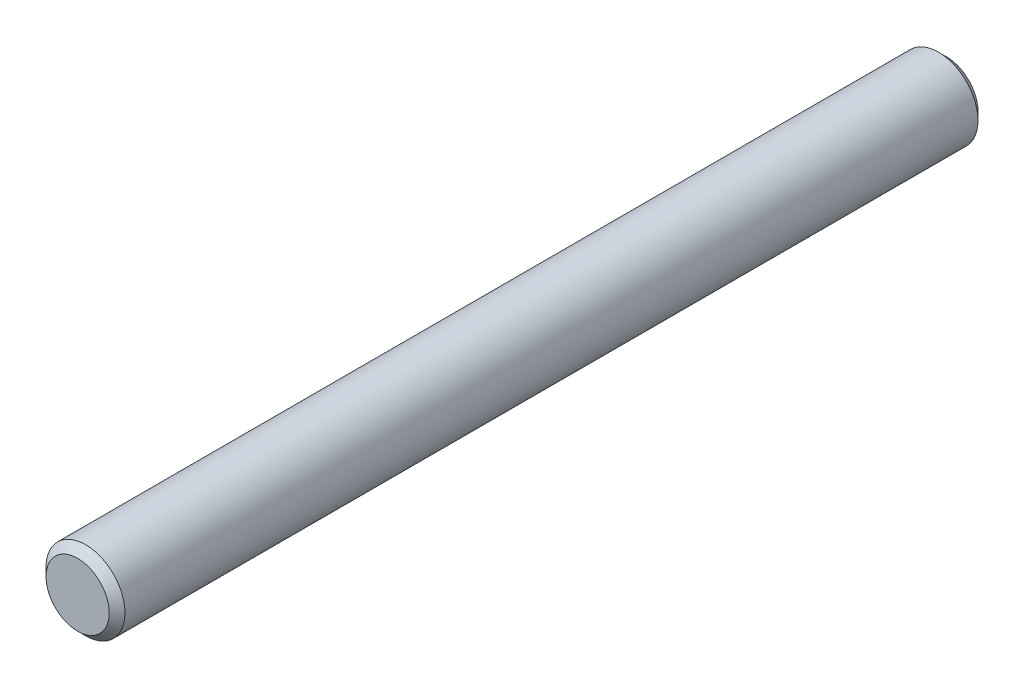
ISO-10303-21;
HEADER;
FILE_DESCRIPTION(('STEP AP214'),'2;1');
FILE_NAME('part.step','',(''),(''),'','','');
FILE_SCHEMA(('AUTOMOTIVE_DESIGN { 1 0 10303 214 1 1 1 1 }'));
ENDSEC;
DATA;
#1=APPLICATION_CONTEXT('core data for automotive mechanical design processes');
#2=APPLICATION_PROTOCOL_DEFINITION('international standard','automotive_design',2000,#1);
#3=PRODUCT_CONTEXT('',#1,'mechanical');
#4=PRODUCT('Part','Part','',(#3));
#5=PRODUCT_RELATED_PRODUCT_CATEGORY('part','',(#4));
#6=PRODUCT_DEFINITION_FORMATION('','',#4);
#7=PRODUCT_DEFINITION_CONTEXT('part definition',#1,'design');
#8=PRODUCT_DEFINITION('design','',#6,#7);
#9=PRODUCT_DEFINITION_SHAPE('','',#8);
#10=(LENGTH_UNIT() NAMED_UNIT(*) SI_UNIT(.MILLI.,.METRE.));
#11=(NAMED_UNIT(*) PLANE_ANGLE_UNIT() SI_UNIT($,.RADIAN.));
#12=(NAMED_UNIT(*) SI_UNIT($,.STERADIAN.) SOLID_ANGLE_UNIT());
#13=UNCERTAINTY_MEASURE_WITH_UNIT(LENGTH_MEASURE(1.E-05),#10,'distance_accuracy_value','');
#14=(GEOMETRIC_REPRESENTATION_CONTEXT(3) GLOBAL_UNCERTAINTY_ASSIGNED_CONTEXT((#13)) GLOBAL_UNIT_ASSIGNED_CONTEXT((#10,
#11,#12)) REPRESENTATION_CONTEXT('',''));
#15=CARTESIAN_POINT('',(0.,0.,0.));
#16=DIRECTION('',(0.,0.,1.));
#17=DIRECTION('',(1.,0.,0.));
#18=AXIS2_PLACEMENT_3D('',#15,#16,#17);
#19=CARTESIAN_POINT('',(0.,0.,27.5));
#20=DIRECTION('',(0.,0.,-1.));
#21=DIRECTION('',(-1.,0.,0.));
#22=AXIS2_PLACEMENT_3D('',#19,#20,#21);
#23=CYLINDRICAL_SURFACE('',#22,2.5);
#24=CARTESIAN_POINT('',(0.,0.,-27.));
#25=DIRECTION('',(0.,0.,1.));
#26=DIRECTION('',(1.,0.,0.));
#27=AXIS2_PLACEMENT_3D('',#24,#25,#26);
#28=CIRCLE('',#27,2.5);
#29=CARTESIAN_POINT('',(2.5,0.,-27.));
#30=VERTEX_POINT('',#29);
#31=EDGE_CURVE('E52',#30,#30,#28,.T.);
#32=ORIENTED_EDGE('',*,*,#31,.T.);
#33=EDGE_LOOP('',(#32));
#34=FACE_BOUND('',#33,.T.);
#35=CARTESIAN_POINT('',(0.,0.,27.));
#36=DIRECTION('',(0.,0.,1.));
#37=DIRECTION('',(1.,0.,0.));
#38=AXIS2_PLACEMENT_3D('',#35,#36,#37);
#39=CIRCLE('',#38,2.5);
#40=CARTESIAN_POINT('',(2.5,0.,27.));
#41=VERTEX_POINT('',#40);
#42=EDGE_CURVE('E60',#41,#41,#39,.F.);
#43=ORIENTED_EDGE('',*,*,#42,.T.);
#44=EDGE_LOOP('',(#43));
#45=FACE_BOUND('',#44,.T.);
#46=ADVANCED_FACE('F41',(#34,#45),#23,.T.);
#47=CARTESIAN_POINT('',(0.,0.,27.5));
#48=DIRECTION('',(0.,0.,1.));
#49=DIRECTION('',(1.,0.,0.));
#50=AXIS2_PLACEMENT_3D('',#47,#48,#49);
#51=PLANE('',#50);
#52=CARTESIAN_POINT('',(0.,0.,27.5));
#53=DIRECTION('',(0.,0.,1.));
#54=DIRECTION('',(1.,0.,0.));
#55=AXIS2_PLACEMENT_3D('',#52,#53,#54);
#56=CIRCLE('',#55,1.99999999999998);
#57=CARTESIAN_POINT('',(1.99999999999998,0.,27.5));
#58=VERTEX_POINT('',#57);
#59=EDGE_CURVE('E10',#58,#58,#56,.T.);
#60=ORIENTED_EDGE('',*,*,#59,.T.);
#61=EDGE_LOOP('',(#60));
#62=FACE_BOUND('',#61,.T.);
#63=ADVANCED_FACE('F71',(#62),#51,.T.);
#64=CARTESIAN_POINT('',(0.,0.,-27.5));
#65=DIRECTION('',(0.,0.,1.));
#66=DIRECTION('',(1.,0.,0.));
#67=AXIS2_PLACEMENT_3D('',#64,#65,#66);
#68=PLANE('',#67);
#69=CARTESIAN_POINT('',(0.,0.,-27.5));
#70=DIRECTION('',(0.,0.,1.));
#71=DIRECTION('',(1.,0.,0.));
#72=AXIS2_PLACEMENT_3D('',#69,#70,#71);
#73=CIRCLE('',#72,2.);
#74=CARTESIAN_POINT('',(2.,0.,-27.5));
#75=VERTEX_POINT('',#74);
#76=EDGE_CURVE('E47',#75,#75,#73,.F.);
#77=ORIENTED_EDGE('',*,*,#76,.T.);
#78=EDGE_LOOP('',(#77));
#79=FACE_BOUND('',#78,.T.);
#80=ADVANCED_FACE('F69',(#79),#68,.F.);
#81=CARTESIAN_POINT('',(0.,0.,-27.));
#82=DIRECTION('',(0.,0.,1.));
#83=DIRECTION('',(1.,0.,0.));
#84=AXIS2_PLACEMENT_3D('',#81,#82,#83);
#85=CONICAL_SURFACE('',#84,2.5,0.785398163397453);
#86=ORIENTED_EDGE('',*,*,#76,.F.);
#87=EDGE_LOOP('',(#86));
#88=FACE_BOUND('',#87,.T.);
#89=ORIENTED_EDGE('',*,*,#31,.F.);
#90=EDGE_LOOP('',(#89));
#91=FACE_BOUND('',#90,.T.);
#92=ADVANCED_FACE('F66',(#88,#91),#85,.T.);
#93=CARTESIAN_POINT('',(0.,0.,27.5));
#94=DIRECTION('',(0.,0.,-1.));
#95=DIRECTION('',(-1.,0.,0.));
#96=AXIS2_PLACEMENT_3D('',#93,#94,#95);
#97=CONICAL_SURFACE('',#96,1.99999999999998,0.785398163397453);
#98=ORIENTED_EDGE('',*,*,#42,.F.);
#99=EDGE_LOOP('',(#98));
#100=FACE_BOUND('',#99,.T.);
#101=ORIENTED_EDGE('',*,*,#59,.F.);
#102=EDGE_LOOP('',(#101));
#103=FACE_BOUND('',#102,.T.);
#104=ADVANCED_FACE('F42',(#100,#103),#97,.T.);
#105=CLOSED_SHELL('',(#46,#63,#80,#92,#104));
#106=MANIFOLD_SOLID_BREP('B2',#105);
#107=ADVANCED_BREP_SHAPE_REPRESENTATION('',(#18,#106),#14);
#108=SHAPE_DEFINITION_REPRESENTATION(#9,#107);
ENDSEC;
END-ISO-10303-21;
